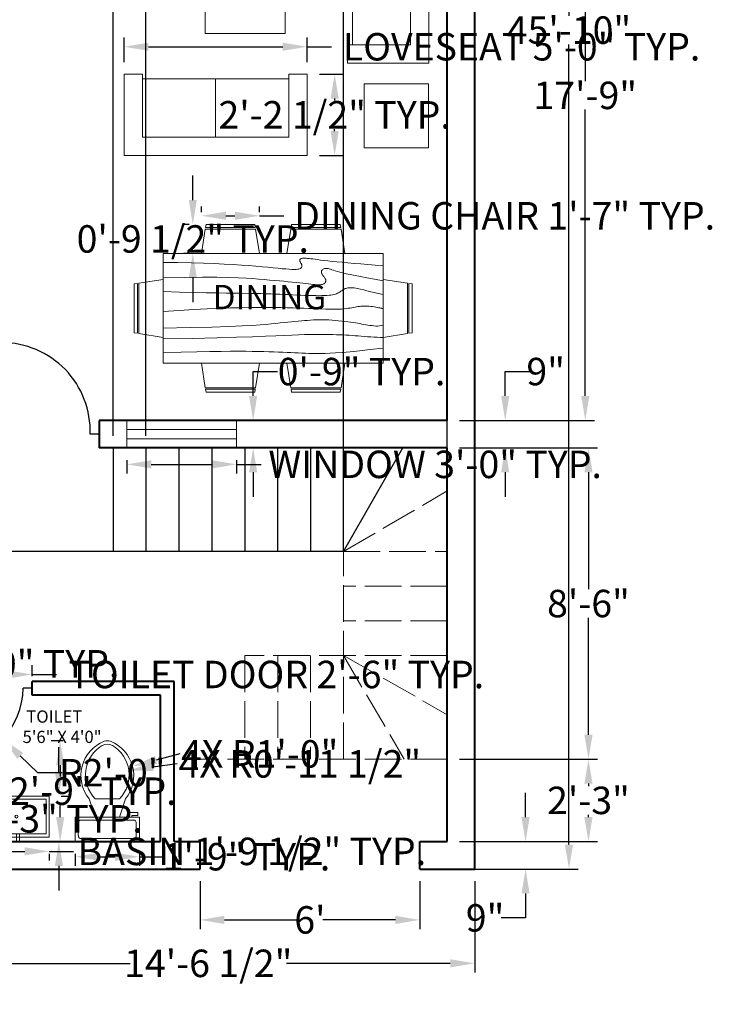
# Model space of a CAD drawing. Units: inches. Extents: x 927 to 1540, y 259 to 890.
# Tile 3 of 4: x 1265 to 1492, y 259 to 582. Entities that reach past the tile are written whole.
import ezdxf

# ---------------------------------------------------------------- set-up
doc = ezdxf.new("R2010")
doc.units = ezdxf.units.IN
doc.header["$MEASUREMENT"] = 0
doc.linetypes.add('ACAD_ISO02W100', pattern=[15, 12, -3])
for name, color, linetype, lineweight in [('A-ANNO-DIMS', 2, 'Continuous', 18), ('A-AREA-IDEN', 7, 'Continuous', 25), ('A-DOOR', 3, 'Continuous', 25), ('A-FLOR-FIXT', 9, 'Continuous', 18), ('A-FLOR-STRS', 7, 'Continuous', 25), ('A-FLOR-STRS-OVHD', 8, 'ACAD_ISO02W100', 18), ('A-FURN', 8, 'Continuous', 18), ('A-GLAZ', 4, 'Continuous', 18), ('A-WALL', 7, 'Continuous', 40)]:
    doc.layers.add(name, color=color, linetype=linetype, lineweight=lineweight)
doc.styles.get("Standard").update_dxf_attribs({"font": 'arial.ttf'})
doc.dimstyles.get("Standard").update_dxf_attribs({"dimtxt": 9, "dimasz": 8, "dimexe": 3, "dimexo": 4, "dimgap": 0.09, "dimtad": 0, "dimtih": 1, "dimtoh": 1, "dimdec": 0, "dimzin": 0, "dimdsep": 46, "dimlunit": 3, "dimtxsty": 'Standard', "dimcen": 0.09, "dimadec": 0, "dimazin": 0, "dimtfac": 1, "dimtdec": 0, "dimtofl": 0, "dimtmove": 0, "dimatfit": 3, "dimfxl": 1, "dimtolj": 1, "dimtzin": 0, "dimarcsym": 0})

# ---------------------------------------------------------------- blocks, each defined once
blk = doc.blocks.new('*D7')
at = {"layer": 'A-ANNO-DIMS', "color": 0, "lineweight": -2, "transparency": 16777216}
for p, q in [((1431.15, 320.39), (1431.15, 328.39)), ((1409.48, 312.39), (1434.15, 312.39)), ((1409.48, 303.39), (1434.15, 303.39)), ((1431.15, 295.39), (1431.15, 287.39)), ((1431.15, 287.39), (1423.15, 287.39))]:
    blk.add_line(p, q, dxfattribs=at)
at = {"layer": 'A-ANNO-DIMS', "color": 0, "lineweight": 100, "transparency": 16777216}
for points in [[(1429.81, 320.39), (1432.48, 320.39), (1431.15, 312.39)], [(1429.81, 295.39), (1432.48, 295.39), (1431.15, 303.39)]]:
    blk.add_solid(points, dxfattribs=at)
at = {"layer": 'Defpoints', "color": 0, "lineweight": 100, "transparency": 16777216}
for p in [(1405.48, 312.39), (1405.48, 303.39), (1431.15, 303.39)]:
    blk.add_point(p, dxfattribs=at)
at = {"layer": 'A-ANNO-DIMS', "color": 0, "transparency": 16777216, "insert": (1417.89, 287.39), "char_height": 9, "attachment_point": 5}
blk.add_mtext('\\A1;9"', dxfattribs=at)
blk = doc.blocks.new('*D8')
at = {"layer": 'A-ANNO-DIMS', "color": 0, "lineweight": -2, "transparency": 16777216}
for p, q in [((1418.48, 339.39), (1454.76, 339.39)), ((1451.76, 331.39), (1451.76, 330.58)), ((1451.76, 320.39), (1451.76, 321.2)), ((1418.48, 312.39), (1454.76, 312.39))]:
    blk.add_line(p, q, dxfattribs=at)
at = {"layer": 'A-ANNO-DIMS', "color": 0, "lineweight": 100, "transparency": 16777216}
for points in [[(1450.42, 331.39), (1453.09, 331.39), (1451.76, 339.39)], [(1450.42, 320.39), (1453.09, 320.39), (1451.76, 312.39)]]:
    blk.add_solid(points, dxfattribs=at)
at = {"layer": 'Defpoints', "color": 0, "lineweight": 100, "transparency": 16777216}
for p in [(1414.48, 339.39), (1451.76, 339.39), (1414.48, 312.39)]:
    blk.add_point(p, dxfattribs=at)
at = {"layer": 'A-ANNO-DIMS', "color": 0, "transparency": 16777216, "insert": (1451.76, 325.89), "char_height": 9, "attachment_point": 5}
blk.add_mtext('\\A1;2\'-3"', dxfattribs=at)
blk = doc.blocks.new('*D9')
at = {"layer": 'A-ANNO-DIMS', "color": 0, "lineweight": -2, "transparency": 16777216}
for p, q in [((1409.48, 441.39), (1454.76, 441.39)), ((1451.76, 433.39), (1451.76, 395.08)), ((1451.76, 347.39), (1451.76, 385.71)), ((1409.48, 339.39), (1454.76, 339.39))]:
    blk.add_line(p, q, dxfattribs=at)
at = {"layer": 'A-ANNO-DIMS', "color": 0, "lineweight": 100, "transparency": 16777216}
for points in [[(1450.43, 433.39), (1453.1, 433.39), (1451.76, 441.39)], [(1450.43, 347.39), (1453.1, 347.39), (1451.76, 339.39)]]:
    blk.add_solid(points, dxfattribs=at)
at = {"layer": 'Defpoints', "color": 0, "lineweight": 100, "transparency": 16777216}
for p in [(1405.48, 441.39), (1451.76, 441.39), (1405.48, 339.39)]:
    blk.add_point(p, dxfattribs=at)
at = {"layer": 'A-ANNO-DIMS', "color": 0, "transparency": 16777216, "insert": (1451.76, 390.39), "char_height": 9, "attachment_point": 5}
blk.add_mtext('\\A1;8\'-6"', dxfattribs=at)
blk = doc.blocks.new('*D10')
at = {"layer": 'A-ANNO-DIMS', "color": 0, "lineweight": -2, "transparency": 16777216}
for p, q in [((1424.47, 458.39), (1424.47, 466.39)), ((1424.47, 466.39), (1432.47, 466.39)), ((1409.48, 450.39), (1427.47, 450.39)), ((1409.48, 441.39), (1427.47, 441.39)), ((1424.47, 433.39), (1424.47, 425.39))]:
    blk.add_line(p, q, dxfattribs=at)
at = {"layer": 'A-ANNO-DIMS', "color": 0, "lineweight": 100, "transparency": 16777216}
for points in [[(1423.14, 458.39), (1425.81, 458.39), (1424.47, 450.39)], [(1423.14, 433.39), (1425.81, 433.39), (1424.47, 441.39)]]:
    blk.add_solid(points, dxfattribs=at)
at = {"layer": 'Defpoints', "color": 0, "lineweight": 100, "transparency": 16777216}
for p in [(1405.48, 450.39), (1424.47, 450.39), (1405.48, 441.39)]:
    blk.add_point(p, dxfattribs=at)
at = {"layer": 'A-ANNO-DIMS', "color": 0, "transparency": 16777216, "insert": (1437.74, 466.39), "char_height": 9, "attachment_point": 5}
blk.add_mtext('\\A1;9"', dxfattribs=at)
blk = doc.blocks.new('*D11')
at = {"layer": 'A-ANNO-DIMS', "color": 0, "lineweight": -2, "transparency": 16777216}
for p, q in [((1409.48, 663.39), (1453.72, 663.39)), ((1450.72, 655.39), (1450.72, 561.58)), ((1450.72, 458.39), (1450.72, 552.21)), ((1418.48, 450.39), (1453.72, 450.39))]:
    blk.add_line(p, q, dxfattribs=at)
at = {"layer": 'A-ANNO-DIMS', "color": 0, "lineweight": 100, "transparency": 16777216}
for points in [[(1449.39, 655.39), (1452.05, 655.39), (1450.72, 663.39)], [(1449.39, 458.39), (1452.05, 458.39), (1450.72, 450.39)]]:
    blk.add_solid(points, dxfattribs=at)
at = {"layer": 'Defpoints', "color": 0, "lineweight": 100, "transparency": 16777216}
for p in [(1405.48, 663.39), (1450.72, 663.39), (1414.48, 450.39)]:
    blk.add_point(p, dxfattribs=at)
at = {"layer": 'A-ANNO-DIMS', "color": 0, "transparency": 16777216, "insert": (1450.72, 556.89), "char_height": 9, "attachment_point": 5}
blk.add_mtext('\\A1;17\'-9"', dxfattribs=at)
blk = doc.blocks.new('*D15')
at = {"layer": 'A-ANNO-DIMS', "color": 0, "lineweight": -2, "transparency": 16777216}
for p, q in [((1324.48, 299.39), (1324.48, 283.73)), ((1396.48, 299.39), (1396.48, 283.73)), ((1332.48, 286.73), (1356.22, 286.73)), ((1388.48, 286.73), (1364.73, 286.73))]:
    blk.add_line(p, q, dxfattribs=at)
at = {"layer": 'A-ANNO-DIMS', "color": 0, "lineweight": 100, "transparency": 16777216}
for points in [[(1332.48, 288.06), (1332.48, 285.39), (1324.48, 286.73)], [(1388.48, 288.06), (1388.48, 285.39), (1396.48, 286.73)]]:
    blk.add_solid(points, dxfattribs=at)
at = {"layer": 'Defpoints', "color": 0, "lineweight": 100, "transparency": 16777216}
for p in [(1324.48, 303.39), (1396.48, 303.39), (1396.48, 286.73)]:
    blk.add_point(p, dxfattribs=at)
at = {"layer": 'A-ANNO-DIMS', "color": 0, "transparency": 16777216, "insert": (1360.48, 286.73), "char_height": 9, "attachment_point": 5}
blk.add_mtext("\\A1;6'", dxfattribs=at)
blk = doc.blocks.new('DOOR-SINGLE-36-OPENING')
for p, q in [((3, 0), (3, 30)), ((3, 30), (4, 30)), ((4, 30), (4, 0)), ((0, 0), (3, 0)), ((4, 0), (3, 0)), ((36, 0), (33, 0))]:
    blk.add_line(p, q)
blk.add_arc((4, 0.98), 29.02, 358.058, 90)
blk = doc.blocks.new('DOOR-SINGLE-30-OPENING')
for p, q in [((0, 24), (3, 24)), ((3, 24), (3, 0)), ((4, 24), (3, 24)), ((4, 0), (4, 24)), ((30, 24), (27, 24)), ((3, 0), (4, 0))]:
    blk.add_line(p, q)
blk.add_arc((2.98, 24), 24.02, 272.4378, 0)
blk = doc.blocks.new('SOFA-LOVESEAT-60')
for p, q in [((26.6182, 60.00004), (26.6182, 0)), ((0, 54.00004), (1.558, 54.00004)), ((1.558, 54.00004), (1.558, 6)), ((1.558, 54.00004), (20.6182, 53.99984)), ((20.6182, 53.99984), (20.6182, 6.00018)), ((1.558, 30.00004), (20.6182, 30.00004)), ((0, 6), (1.558, 6)), ((20.6182, 6.00018), (1.558, 6))]:
    blk.add_line(p, q)
for points in [[(0, 54.00004), (0, 60.00004), (26.6182, 60.00004)], [(26.6182, 0), (0, 0), (0, 6)]]:
    blk.add_lwpolyline(points)
blk = doc.blocks.new('CHAIR-DINING')
for p, q in [((1.2504, 8.00297), (0, 0)), ((1.2543, 8.00238), (17.7239, 8.00238)), ((1.4847, 9.50238), (1.3285, 8.5028)), ((17.6431, 8.50238), (1.3313, 8.50238)), ((1.4847, 9.50238), (17.4847, 9.50238)), ((17.641, 8.50204), (17.4847, 9.50238)), ((18.9695, 0), (17.7192, 8.00164))]:
    blk.add_line(p, q)
blk = doc.blocks.new('WC-TANK-TYPE')
for p, q in [((23.5, 17.5), (23.5, 20.5)), ((23.5, 20.5), (24.5, 20.5)), ((24.5, 20.5), (24.5, 18.5)), ((25, 14.5), (19, 16.5)), ((25, 17.5), (23.5, 17.5)), ((24.5, 18.5), (25, 18.5)), ((19, 6.5), (19, 14.5)), ((25, 6.5), (19, 4.5)), ((27, 1), (31, 1))]:
    blk.add_line(p, q)
blk.add_lwpolyline([(25, 0), (33, 0), (33, 21), (25, 21)], close=True)
for points in [[(31, 20), (27, 20)], [(26, 19), (26, 2)], [(32, 2), (32, 19)]]:
    blk.add_lwpolyline(points)
for centre, radius, start, end in [((26.87, 19.12), 0.884, 81.8699, 188.1301), ((31.12, 19.12), 0.884, 351.8699, 98.1301), ((11.42, 6.98), 12.17, 51.4691, 157.9714), ((11.18, 6.3), 11.33, 46.3677, 148.9468), ((4, 10.5), 4, 164.8605, 195.1395), ((5.12, 10.5), 4, 155.7318, 204.2682), ((11.42, 14.02), 12.17, 202.0284, 308.5307), ((11.18, 14.7), 11.33, 211.053, 313.6321), ((26.87, 1.88), 0.884, 171.8699, 278.1301), ((31.12, 1.88), 0.884, 261.8699, 8.1301)]:
    blk.add_arc(centre, radius, start, end)
blk = doc.blocks.new('LAVATORY-RECTANGULAR')
for p, q in [((10.69, 2.5), (10.69, 0)), ((11.69, 2.5), (11.69, 0))]:
    blk.add_line(p, q)
for points in [[(0, 1.5), (21.39, 1.5), (21.39, 14.9), (0, 14.9)], [(1, 2.5), (20.39, 2.5), (20.39, 13.9), (1, 13.9)]]:
    blk.add_lwpolyline(points, close=True)
blk.add_circle((10.69, 8.2), 0.491)
blk = doc.blocks.new('WINDOW-36')
for p, q in [((0, 9), (0, 0)), ((36, 9), (36, 0)), ((0, 6), (36, 6)), ((0, 3), (36, 3))]:
    blk.add_line(p, q)
blk = doc.blocks.new('*D30')
at = {"layer": 'A-ANNO-DIMS', "color": 0, "lineweight": -2, "transparency": 16777216}
for p, q in [((1324.96, 518.6), (1324.96, 520.44)), ((1343.93, 518.6), (1343.93, 520.44)), ((1332.96, 517.44), (1335.93, 517.44)), ((1343.93, 517.44), (1351.93, 517.44))]:
    blk.add_line(p, q, dxfattribs=at)
at = {"layer": 'A-ANNO-DIMS', "color": 0, "lineweight": 100, "transparency": 16777216}
for points in [[(1332.96, 518.78), (1332.96, 516.11), (1324.96, 517.44)], [(1335.93, 518.78), (1335.93, 516.11), (1343.93, 517.44)]]:
    blk.add_solid(points, dxfattribs=at)
at = {"layer": 'Defpoints', "color": 0, "lineweight": 100, "transparency": 16777216}
for p in [(1343.93, 517.44), (1324.96, 514.6), (1343.93, 514.6)]:
    blk.add_point(p, dxfattribs=at)
at = {"layer": 'A-ANNO-DIMS', "color": 0, "transparency": 16777216, "insert": (1424.28, 517.44), "char_height": 9, "attachment_point": 5}
blk.add_mtext('\\A1;DINING CHAIR 1\'-7" TYP.', dxfattribs=at)
blk = doc.blocks.new('*D31')
at = {"layer": 'A-ANNO-DIMS', "color": 0, "lineweight": -2, "transparency": 16777216}
for p, q in [((1322.11, 522.6), (1322.11, 530.6)), ((1320.96, 514.6), (1319.11, 514.6)), ((1320.96, 505.1), (1319.11, 505.1)), ((1322.11, 497.1), (1322.11, 489.1))]:
    blk.add_line(p, q, dxfattribs=at)
at = {"layer": 'A-ANNO-DIMS', "color": 0, "lineweight": 100, "transparency": 16777216}
for points in [[(1320.78, 522.6), (1323.44, 522.6), (1322.11, 514.6)], [(1320.78, 497.1), (1323.44, 497.1), (1322.11, 505.1)]]:
    blk.add_solid(points, dxfattribs=at)
at = {"layer": 'Defpoints', "color": 0, "lineweight": 100, "transparency": 16777216}
for p in [(1322.11, 514.6), (1324.96, 514.6), (1324.96, 505.1)]:
    blk.add_point(p, dxfattribs=at)
at = {"layer": 'A-ANNO-DIMS', "color": 0, "transparency": 16777216, "insert": (1322.11, 509.85), "char_height": 9, "attachment_point": 5}
blk.add_mtext('\\A1;0\'-9 1/2" TYP.', dxfattribs=at)
blk = doc.blocks.new('*D34')
at = {"layer": 'A-ANNO-DIMS', "color": 0, "lineweight": -2, "transparency": 16777216}
for p, q in [((1239.48, 366.64), (1239.48, 370.14)), ((1269.48, 366.64), (1269.48, 370.14)), ((1247.48, 367.14), (1261.48, 367.14)), ((1269.48, 367.14), (1277.48, 367.14))]:
    blk.add_line(p, q, dxfattribs=at)
at = {"layer": 'A-ANNO-DIMS', "color": 0, "lineweight": 100, "transparency": 16777216}
for points in [[(1247.48, 368.47), (1247.48, 365.81), (1239.48, 367.14)], [(1261.48, 368.47), (1261.48, 365.81), (1269.48, 367.14)]]:
    blk.add_solid(points, dxfattribs=at)
at = {"layer": 'Defpoints', "color": 0, "lineweight": 100, "transparency": 16777216}
for p in [(1269.48, 367.14), (1239.48, 362.64), (1269.48, 362.64)]:
    blk.add_point(p, dxfattribs=at)
at = {"layer": 'A-ANNO-DIMS', "color": 0, "transparency": 16777216, "insert": (1349.47, 367.14), "char_height": 9, "attachment_point": 5}
blk.add_mtext('\\A1;TOILET DOOR 2\'-6" TYP.', dxfattribs=at)
blk = doc.blocks.new('*D35')
at = {"layer": 'A-ANNO-DIMS', "color": 0, "lineweight": -2, "transparency": 16777216}
for p, q in [((1234.98, 362.64), (1234.98, 370.64)), ((1234.98, 370.64), (1242.98, 370.64)), ((1235.48, 362.64), (1231.98, 362.64)), ((1234.98, 346.64), (1234.98, 354.64)), ((1235.48, 338.64), (1231.98, 338.64))]:
    blk.add_line(p, q, dxfattribs=at)
at = {"layer": 'A-ANNO-DIMS', "color": 0, "lineweight": 100, "transparency": 16777216}
for points in [[(1233.64, 354.64), (1236.31, 354.64), (1234.98, 362.64)], [(1233.64, 346.64), (1236.31, 346.64), (1234.98, 338.64)]]:
    blk.add_solid(points, dxfattribs=at)
at = {"layer": 'Defpoints', "color": 0, "lineweight": 100, "transparency": 16777216}
for p in [(1234.98, 362.64), (1239.48, 362.64), (1239.48, 338.64)]:
    blk.add_point(p, dxfattribs=at)
at = {"layer": 'A-ANNO-DIMS', "color": 0, "transparency": 16777216, "insert": (1270.57, 370.64), "char_height": 9, "attachment_point": 5}
blk.add_mtext('\\A1;2\'-0" TYP.', dxfattribs=at)
blk = doc.blocks.new('*D36')
at = {"layer": 'A-ANNO-DIMS', "color": 0, "lineweight": -2, "transparency": 16777216}
for p, q in [((1299.59, 567.82), (1299.59, 575.82)), ((1359.59, 567.82), (1359.59, 575.82)), ((1307.59, 572.82), (1351.59, 572.82)), ((1359.59, 572.82), (1367.59, 572.82))]:
    blk.add_line(p, q, dxfattribs=at)
at = {"layer": 'A-ANNO-DIMS', "color": 0, "lineweight": 100, "transparency": 16777216}
for points in [[(1307.59, 574.16), (1307.59, 571.49), (1299.59, 572.82)], [(1351.59, 574.16), (1351.59, 571.49), (1359.59, 572.82)]]:
    blk.add_solid(points, dxfattribs=at)
at = {"layer": 'Defpoints', "color": 0, "lineweight": 100, "transparency": 16777216}
for p in [(1359.59, 572.82), (1299.59, 563.82), (1359.59, 563.82)]:
    blk.add_point(p, dxfattribs=at)
at = {"layer": 'A-ANNO-DIMS', "color": 0, "transparency": 16777216, "insert": (1429.85, 572.82), "char_height": 9, "attachment_point": 5}
blk.add_mtext('\\A1;LOVESEAT 5\'-0" TYP.', dxfattribs=at)
blk = doc.blocks.new('*D37')
at = {"layer": 'A-ANNO-DIMS', "color": 0, "lineweight": -2, "transparency": 16777216}
for p, q in [((1363.59, 563.82), (1371.59, 563.82)), ((1368.59, 555.82), (1368.59, 555.26)), ((1368.59, 545.21), (1368.59, 545.77)), ((1363.59, 537.21), (1371.59, 537.21))]:
    blk.add_line(p, q, dxfattribs=at)
at = {"layer": 'A-ANNO-DIMS', "color": 0, "lineweight": 100, "transparency": 16777216}
for points in [[(1367.26, 555.82), (1369.93, 555.82), (1368.59, 563.82)], [(1367.26, 545.21), (1369.93, 545.21), (1368.59, 537.21)]]:
    blk.add_solid(points, dxfattribs=at)
at = {"layer": 'Defpoints', "color": 0, "lineweight": 100, "transparency": 16777216}
for p in [(1359.59, 563.82), (1359.59, 537.21), (1368.59, 537.21)]:
    blk.add_point(p, dxfattribs=at)
at = {"layer": 'A-ANNO-DIMS', "color": 0, "transparency": 16777216, "insert": (1368.59, 550.52), "char_height": 9, "attachment_point": 5}
blk.add_mtext('\\A1;2\'-2 1/2" TYP.', dxfattribs=at)
blk = doc.blocks.new('*D44')
at = {"layer": 'A-ANNO-DIMS', "color": 0, "lineweight": -2, "transparency": 16777216}
for p, q in [((1279.6, 345.44), (1275.65, 345.44)), ((1278.65, 337.44), (1278.65, 333.66)), ((1278.65, 320.39), (1278.65, 324.17)), ((1279.6, 312.39), (1275.65, 312.39))]:
    blk.add_line(p, q, dxfattribs=at)
at = {"layer": 'A-ANNO-DIMS', "color": 0, "lineweight": 100, "transparency": 16777216}
for points in [[(1277.31, 337.44), (1279.98, 337.44), (1278.65, 345.44)], [(1277.31, 320.39), (1279.98, 320.39), (1278.65, 312.39)]]:
    blk.add_solid(points, dxfattribs=at)
at = {"layer": 'Defpoints', "color": 0, "lineweight": 100, "transparency": 16777216}
for p in [(1283.6, 345.44), (1278.65, 312.39), (1283.6, 312.39)]:
    blk.add_point(p, dxfattribs=at)
at = {"layer": 'A-ANNO-DIMS', "color": 0, "transparency": 16777216, "insert": (1278.65, 328.91), "char_height": 9, "attachment_point": 5}
blk.add_mtext('\\A1;WC 2\'-9" TYP.', dxfattribs=at)
blk = doc.blocks.new('*D45')
at = {"layer": 'A-ANNO-DIMS', "color": 0, "lineweight": -2, "transparency": 16777216}
for p, q in [((1283.6, 308.39), (1283.6, 304.43)), ((1291.6, 307.43), (1296.6, 307.43)), ((1304.6, 308.39), (1304.6, 304.43)), ((1304.6, 307.43), (1312.6, 307.43))]:
    blk.add_line(p, q, dxfattribs=at)
at = {"layer": 'A-ANNO-DIMS', "color": 0, "lineweight": 100, "transparency": 16777216}
for points in [[(1291.6, 308.77), (1291.6, 306.1), (1283.6, 307.43)], [(1296.6, 308.77), (1296.6, 306.1), (1304.6, 307.43)]]:
    blk.add_solid(points, dxfattribs=at)
at = {"layer": 'Defpoints', "color": 0, "lineweight": 100, "transparency": 16777216}
for p in [(1283.6, 312.39), (1304.6, 312.39), (1304.6, 307.43)]:
    blk.add_point(p, dxfattribs=at)
at = {"layer": 'A-ANNO-DIMS', "color": 0, "transparency": 16777216, "insert": (1339.7, 307.43), "char_height": 9, "attachment_point": 5}
blk.add_mtext('\\A1;1\'-9" TYP.', dxfattribs=at)
blk = doc.blocks.new('*D46')
at = {"layer": 'A-ANNO-DIMS', "color": 0, "lineweight": -2, "transparency": 16777216}
for p, q in [((1253.64, 308.39), (1253.64, 306.18)), ((1261.64, 309.18), (1267.03, 309.18)), ((1275.03, 309.18), (1283.03, 309.18)), ((1275.03, 308.39), (1275.03, 306.18))]:
    blk.add_line(p, q, dxfattribs=at)
at = {"layer": 'A-ANNO-DIMS', "color": 0, "lineweight": 100, "transparency": 16777216}
for points in [[(1261.64, 310.52), (1261.64, 307.85), (1253.64, 309.18)], [(1267.03, 310.52), (1267.03, 307.85), (1275.03, 309.18)]]:
    blk.add_solid(points, dxfattribs=at)
at = {"layer": 'Defpoints', "color": 0, "lineweight": 100, "transparency": 16777216}
for p in [(1253.64, 312.39), (1275.03, 312.39), (1275.03, 309.18)]:
    blk.add_point(p, dxfattribs=at)
at = {"layer": 'A-ANNO-DIMS', "color": 0, "transparency": 16777216, "insert": (1341.45, 309.18), "char_height": 9, "attachment_point": 5}
blk.add_mtext('\\A1;BASIN 1\'-9 1/2" TYP.', dxfattribs=at)
blk = doc.blocks.new('*D47')
at = {"layer": 'A-ANNO-DIMS', "color": 0, "lineweight": -2, "transparency": 16777216}
for p, q in [((1278.23, 335.29), (1278.23, 343.29)), ((1279.03, 327.29), (1281.23, 327.29)), ((1279.03, 312.39), (1281.23, 312.39)), ((1278.23, 304.39), (1278.23, 296.39))]:
    blk.add_line(p, q, dxfattribs=at)
at = {"layer": 'A-ANNO-DIMS', "color": 0, "lineweight": 100, "transparency": 16777216}
for points in [[(1276.9, 335.29), (1279.57, 335.29), (1278.23, 327.29)], [(1276.9, 304.39), (1279.57, 304.39), (1278.23, 312.39)]]:
    blk.add_solid(points, dxfattribs=at)
at = {"layer": 'Defpoints', "color": 0, "lineweight": 100, "transparency": 16777216}
for p in [(1275.03, 327.29), (1278.23, 327.29), (1275.03, 312.39)]:
    blk.add_point(p, dxfattribs=at)
at = {"layer": 'A-ANNO-DIMS', "color": 0, "transparency": 16777216, "insert": (1278.23, 319.84), "char_height": 9, "attachment_point": 5}
blk.add_mtext('\\A1;1\'-3" TYP.', dxfattribs=at)
blk = doc.blocks.new('*D48')
at = {"layer": 'A-ANNO-DIMS', "color": 0, "lineweight": -2, "transparency": 16777216}
for p, q in [((1300.48, 437.39), (1300.48, 432.99)), ((1308.48, 435.99), (1328.48, 435.99)), ((1336.48, 437.39), (1336.48, 432.99)), ((1336.48, 435.99), (1344.48, 435.99))]:
    blk.add_line(p, q, dxfattribs=at)
at = {"layer": 'A-ANNO-DIMS', "color": 0, "lineweight": 100, "transparency": 16777216}
for points in [[(1308.48, 437.32), (1308.48, 434.66), (1300.48, 435.99)], [(1328.48, 437.32), (1328.48, 434.66), (1336.48, 435.99)]]:
    blk.add_solid(points, dxfattribs=at)
at = {"layer": 'Defpoints', "color": 0, "lineweight": 100, "transparency": 16777216}
for p in [(1300.48, 441.39), (1336.48, 441.39), (1336.48, 435.99)]:
    blk.add_point(p, dxfattribs=at)
at = {"layer": 'A-ANNO-DIMS', "color": 0, "transparency": 16777216, "insert": (1401.51, 435.99), "char_height": 9, "attachment_point": 5}
blk.add_mtext('\\A1;WINDOW 3\'-0" TYP.', dxfattribs=at)
blk = doc.blocks.new('*D49')
at = {"layer": 'A-ANNO-DIMS', "color": 0, "lineweight": -2, "transparency": 16777216}
for p, q in [((1341.88, 458.39), (1341.88, 466.39)), ((1341.88, 466.39), (1349.88, 466.39)), ((1340.48, 450.39), (1344.88, 450.39)), ((1340.48, 441.39), (1344.88, 441.39)), ((1341.88, 433.39), (1341.88, 425.39))]:
    blk.add_line(p, q, dxfattribs=at)
at = {"layer": 'A-ANNO-DIMS', "color": 0, "lineweight": 100, "transparency": 16777216}
for points in [[(1340.54, 458.39), (1343.21, 458.39), (1341.88, 450.39)], [(1340.54, 433.39), (1343.21, 433.39), (1341.88, 441.39)]]:
    blk.add_solid(points, dxfattribs=at)
at = {"layer": 'Defpoints', "color": 0, "lineweight": 100, "transparency": 16777216}
for p in [(1336.48, 450.39), (1341.88, 450.39), (1336.48, 441.39)]:
    blk.add_point(p, dxfattribs=at)
at = {"layer": 'A-ANNO-DIMS', "color": 0, "transparency": 16777216, "insert": (1377.4, 466.39), "char_height": 9, "attachment_point": 5}
blk.add_mtext('\\A1;0\'-9" TYP.', dxfattribs=at)
blk = doc.blocks.new('*D51')
at = {"layer": 'A-ANNO-DIMS', "color": 0, "lineweight": -2, "transparency": 16777216}
for p, q in [((1418.48, 853.14), (1448.38, 853.14)), ((1445.38, 845.14), (1445.38, 582.95)), ((1445.38, 311.39), (1445.38, 573.58)), ((1418.48, 303.39), (1448.38, 303.39))]:
    blk.add_line(p, q, dxfattribs=at)
at = {"layer": 'A-ANNO-DIMS', "color": 0, "lineweight": 100, "transparency": 16777216}
for points in [[(1444.04, 845.14), (1446.71, 845.14), (1445.38, 853.14)], [(1444.04, 311.39), (1446.71, 311.39), (1445.38, 303.39)]]:
    blk.add_solid(points, dxfattribs=at)
at = {"layer": 'Defpoints', "color": 0, "lineweight": 100, "transparency": 16777216}
for p in [(1414.48, 853.14), (1445.38, 853.14), (1414.48, 303.39)]:
    blk.add_point(p, dxfattribs=at)
at = {"layer": 'A-ANNO-DIMS', "color": 0, "transparency": 16777216, "insert": (1445.38, 578.27), "char_height": 9, "attachment_point": 5}
blk.add_mtext('\\A1;45\'-10"', dxfattribs=at)
blk = doc.blocks.new('*D52')
at = {"layer": 'A-ANNO-DIMS', "color": 0, "lineweight": -2, "transparency": 16777216}
for p, q in [((1239.89, 299.39), (1239.89, 269.49)), ((1414.48, 299.39), (1414.48, 269.49)), ((1247.89, 272.49), (1301.57, 272.49)), ((1406.48, 272.49), (1352.79, 272.49))]:
    blk.add_line(p, q, dxfattribs=at)
at = {"layer": 'A-ANNO-DIMS', "color": 0, "lineweight": 100, "transparency": 16777216}
for points in [[(1247.89, 273.82), (1247.89, 271.16), (1239.89, 272.49)], [(1406.48, 273.82), (1406.48, 271.16), (1414.48, 272.49)]]:
    blk.add_solid(points, dxfattribs=at)
at = {"layer": 'Defpoints', "color": 0, "lineweight": 100, "transparency": 16777216}
for p in [(1239.89, 303.39), (1414.48, 303.39), (1414.48, 272.49)]:
    blk.add_point(p, dxfattribs=at)
at = {"layer": 'A-ANNO-DIMS', "color": 0, "transparency": 16777216, "insert": (1327.18, 272.49), "char_height": 9, "attachment_point": 5}
blk.add_mtext('\\A1;14\'-6 1/2"', dxfattribs=at)
blk = doc.blocks.new('*D54')
at = {"layer": 'A-ANNO-DIMS', "color": 0, "lineweight": -2, "transparency": 16777216}
for p, q in [((1363.48, 884.04), (1355.48, 884.04)), ((1371.48, 411.39), (1371.48, 887.04)), ((1405.48, 411.39), (1405.48, 887.04)), ((1413.48, 884.04), (1421.48, 884.04))]:
    blk.add_line(p, q, dxfattribs=at)
at = {"layer": 'A-ANNO-DIMS', "color": 0, "lineweight": 100, "transparency": 16777216}
for points in [[(1363.48, 885.38), (1363.48, 882.71), (1371.48, 884.04)], [(1413.48, 885.38), (1413.48, 882.71), (1405.48, 884.04)]]:
    blk.add_solid(points, dxfattribs=at)
at = {"layer": 'Defpoints', "color": 0, "lineweight": 100, "transparency": 16777216}
for p in [(1405.48, 884.04), (1371.48, 407.39), (1405.48, 407.39)]:
    blk.add_point(p, dxfattribs=at)
at = {"layer": 'A-ANNO-DIMS', "color": 0, "transparency": 16777216, "insert": (1388.48, 884.04), "char_height": 9, "attachment_point": 5}
blk.add_mtext('\\A1;2\'-10"', dxfattribs=at)
blk = doc.blocks.new('*D55')
at = {"layer": 'A-ANNO-DIMS', "color": 0, "lineweight": -2, "transparency": 16777216}
for p, q in [((1287.98, 884.04), (1279.98, 884.04)), ((1295.98, 445.39), (1295.98, 887.04)), ((1306.76, 445.39), (1306.76, 887.04)), ((1314.76, 884.04), (1322.76, 884.04))]:
    blk.add_line(p, q, dxfattribs=at)
at = {"layer": 'A-ANNO-DIMS', "color": 0, "lineweight": 100, "transparency": 16777216}
for points in [[(1287.98, 885.38), (1287.98, 882.71), (1295.98, 884.04)], [(1314.76, 885.38), (1314.76, 882.71), (1306.76, 884.04)]]:
    blk.add_solid(points, dxfattribs=at)
at = {"layer": 'Defpoints', "color": 0, "lineweight": 100, "transparency": 16777216}
for p in [(1306.76, 884.04), (1295.98, 441.39), (1306.76, 441.39)]:
    blk.add_point(p, dxfattribs=at)
at = {"layer": 'A-ANNO-DIMS', "color": 0, "transparency": 16777216, "insert": (1338.31, 884.04), "char_height": 9, "attachment_point": 5}
blk.add_mtext('\\A1;0\'-11"', dxfattribs=at)
blk = doc.blocks.new('*D60')
at = {"layer": 'A-ANNO-DIMS', "color": 0, "lineweight": -2, "transparency": 16777216}
for p, q in [((1242.37, 362.64), (1242.55, 362.64)), ((1242.46, 362.55), (1242.46, 362.73)), ((1271.35, 334.95), (1265.58, 340.49)), ((1279.35, 334.95), (1271.35, 334.95))]:
    blk.add_line(p, q, dxfattribs=at)
at = {"layer": 'A-ANNO-DIMS', "color": 0, "lineweight": 100, "transparency": 16777216}
blk.add_solid([(1266.5, 341.45), (1264.65, 339.52), (1259.8, 346.02)], dxfattribs=at)
at = {"layer": 'Defpoints', "color": 0, "lineweight": 100, "transparency": 16777216}
for p in [(1242.46, 362.64), (1259.8, 346.02)]:
    blk.add_point(p, dxfattribs=at)
at = {"layer": 'A-ANNO-DIMS', "color": 0, "transparency": 16777216, "insert": (1295.71, 334.95), "char_height": 9, "attachment_point": 5}
blk.add_mtext('\\A1;R2\'-0"', dxfattribs=at)
blk = doc.blocks.new('*D61')
at = {"layer": 'A-ANNO-DIMS', "color": 0, "lineweight": -2, "transparency": 16777216}
for p, q in [((1317.83, 341.13), (1310.09, 339.1)), ((1290.49, 333.97), (1290.67, 333.97)), ((1290.58, 333.88), (1290.58, 334.06))]:
    blk.add_line(p, q, dxfattribs=at)
at = {"layer": 'A-ANNO-DIMS', "color": 0, "lineweight": 100, "transparency": 16777216}
blk.add_solid([(1309.75, 340.39), (1310.43, 337.81), (1302.35, 337.06)], dxfattribs=at)
at = {"layer": 'Defpoints', "color": 0, "lineweight": 100, "transparency": 16777216}
for p in [(1302.35, 337.06), (1290.58, 333.97)]:
    blk.add_point(p, dxfattribs=at)
at = {"layer": 'A-ANNO-DIMS', "color": 0, "transparency": 16777216, "insert": (1344.04, 341.13), "char_height": 9, "attachment_point": 5}
blk.add_mtext('\\A1;4X R1\'-0"', dxfattribs=at)
blk = doc.blocks.new('*D62')
at = {"layer": 'A-ANNO-DIMS', "color": 0, "lineweight": -2, "transparency": 16777216}
for p, q in [((1316.99, 337.85), (1309.06, 336.78)), ((1289.81, 334.21), (1289.99, 334.21)), ((1289.9, 334.12), (1289.9, 334.3))]:
    blk.add_line(p, q, dxfattribs=at)
at = {"layer": 'A-ANNO-DIMS', "color": 0, "lineweight": 100, "transparency": 16777216}
blk.add_solid([(1308.88, 338.11), (1309.24, 335.46), (1301.13, 335.72)], dxfattribs=at)
at = {"layer": 'Defpoints', "color": 0, "lineweight": 100, "transparency": 16777216}
for p in [(1301.13, 335.72), (1289.9, 334.21)]:
    blk.add_point(p, dxfattribs=at)
at = {"layer": 'A-ANNO-DIMS', "color": 0, "transparency": 16777216, "insert": (1357.18, 337.85), "char_height": 9, "attachment_point": 5}
blk.add_mtext('\\A1;4X R0\'-11 1/2"', dxfattribs=at)

msp = doc.modelspace()

# ---------------------------------------------------------------- linework, layer by layer
at = {"layer": 'A-FLOR-STRS'}
for p, q in [((1291.48, 441.39), (1295.98, 441.39)), ((1295.98, 441.39), (1295.98, 407.39)), ((1306.76, 441.39), (1306.76, 407.39)), ((1317.55, 441.39), (1317.55, 407.39)), ((1328.33, 441.39), (1328.33, 407.39)), ((1339.12, 441.39), (1339.12, 407.39)), ((1349.91, 441.39), (1349.91, 407.39)), ((1360.69, 441.39), (1360.69, 407.39)), ((1371.48, 407.39), (1390.9, 441.39)), ((1371.48, 407.39), (1371.48, 441.39)), ((1371.48, 407.39), (1198.54, 407.39))]:
    msp.add_line(p, q, dxfattribs=at)
at = {"layer": 'A-FLOR-STRS-OVHD'}
for p, q in [((1371.48, 407.39), (1405.48, 427.28)), ((1371.48, 339.39), (1371.48, 407.39)), ((1371.48, 407.39), (1405.48, 407.39)), ((1405.48, 396.05), (1371.48, 396.05)), ((1405.48, 384.72), (1371.48, 384.72)), ((1405.48, 373.39), (1339.16, 373.39)), ((1339.16, 373.39), (1339.16, 339.39)), ((1349.94, 373.39), (1349.94, 339.39)), ((1360.73, 373.39), (1360.73, 339.39)), ((1371.48, 373.39), (1391.36, 339.39)), ((1371.48, 373.39), (1405.48, 353.97)), ((1405.48, 339.39), (1315.98, 339.39))]:
    msp.add_line(p, q, dxfattribs=at)
at = {"layer": 'A-FURN'}
for p, q in [((1384.44, 505.1), (1312.44, 505.1)), ((1312.44, 505.1), (1312.44, 469.1)), ((1384.44, 469.1), (1384.44, 505.1)), ((1312.44, 469.1), (1384.44, 469.1))]:
    msp.add_line(p, q, dxfattribs=at)
for points in [[(1352.35, 577.18), (1326.12, 577.18), (1326.12, 622.34), (1352.35, 622.34)], [(1399.3, 560.68), (1378.3, 560.68), (1378.3, 539.68), (1399.3, 539.68)]]:
    msp.add_lwpolyline(points, close=True, dxfattribs=at)
for points in [[(1312.44, 502.1), (1317.26, 502.08), (1321.63, 502.01), (1325.59, 501.91), (1329.16, 501.79), (1332.4, 501.63), (1335.34, 501.46), (1338.02, 501.28), (1340.48, 501.1), (1342.75, 500.91), (1344.84, 500.73), (1346.75, 500.55), (1348.48, 500.39), (1350.04, 500.24), (1351.42, 500.11), (1352.64, 500.01), (1353.69, 499.93), (1354.58, 499.88), (1355.32, 499.87), (1355.93, 499.88), (1356.42, 499.91), (1356.81, 499.97), (1357.11, 500.05), (1357.35, 500.15), (1357.52, 500.26), (1357.66, 500.4), (1357.76, 500.54), (1357.83, 500.7), (1357.87, 500.86), (1357.88, 501.02), (1357.86, 501.19), (1357.83, 501.35), (1357.77, 501.51), (1357.7, 501.67), (1357.62, 501.81), (1357.54, 501.95), (1357.45, 502.09), (1357.37, 502.22), (1357.29, 502.35), (1357.23, 502.47), (1357.19, 502.6), (1357.17, 502.72), (1357.18, 502.84), (1357.2, 502.96), (1357.25, 503.08), (1357.33, 503.18), (1357.43, 503.28), (1357.55, 503.36), (1357.69, 503.43), (1357.86, 503.49), (1358.06, 503.52), (1358.29, 503.55), (1358.57, 503.56), (1358.89, 503.55), (1359.26, 503.52), (1359.69, 503.49), (1360.19, 503.43), (1360.76, 503.36), (1361.41, 503.28), (1362.16, 503.18), (1363.01, 503.07), (1363.98, 502.94), (1365.08, 502.81), (1366.33, 502.67), (1367.73, 502.51), (1369.3, 502.35), (1371.03, 502.19), (1372.91, 502.01), (1374.95, 501.84), (1377.12, 501.66), (1379.43, 501.47), (1381.88, 501.28), (1384.44, 501.1)], [(1312.44, 497.1), (1319.46, 497.24), (1325.27, 497.3), (1330.02, 497.3), (1333.87, 497.23), (1337, 497.13), (1339.56, 496.99), (1341.73, 496.84), (1343.65, 496.68), (1345.47, 496.53), (1347.22, 496.38), (1348.88, 496.24), (1350.47, 496.11), (1351.97, 495.98), (1353.38, 495.85), (1354.71, 495.72), (1355.94, 495.6), (1357.08, 495.47), (1358.13, 495.35), (1359.09, 495.24), (1359.97, 495.13), (1360.77, 495.03), (1361.48, 494.95), (1362.12, 494.89), (1362.69, 494.85), (1363.19, 494.83), (1363.62, 494.83), (1363.99, 494.85), (1364.32, 494.9), (1364.59, 494.96), (1364.82, 495.05), (1365.02, 495.15), (1365.19, 495.26), (1365.34, 495.4), (1365.45, 495.54), (1365.55, 495.7), (1365.62, 495.87), (1365.66, 496.04), (1365.67, 496.23), (1365.65, 496.41), (1365.61, 496.6), (1365.53, 496.79), (1365.43, 496.97), (1365.31, 497.16), (1365.17, 497.35), (1365.03, 497.54), (1364.88, 497.72), (1364.74, 497.91), (1364.61, 498.1), (1364.49, 498.28), (1364.39, 498.47), (1364.32, 498.66), (1364.26, 498.84), (1364.24, 499.01), (1364.24, 499.19), (1364.28, 499.35), (1364.36, 499.51), (1364.47, 499.67), (1364.62, 499.81), (1364.8, 499.93), (1365.01, 500.04), (1365.25, 500.12), (1365.52, 500.17), (1365.8, 500.19), (1366.11, 500.18), (1366.43, 500.13), (1366.78, 500.04), (1367.18, 499.93), (1367.63, 499.78), (1368.16, 499.61), (1368.77, 499.41), (1369.49, 499.2), (1370.32, 498.97), (1371.28, 498.73), (1372.4, 498.47), (1373.72, 498.18), (1375.27, 497.86), (1377.08, 497.5), (1379.19, 497.09), (1381.63, 496.63), (1384.44, 496.1)], [(1312.44, 492.6), (1317.72, 492.43), (1322.37, 492.31), (1326.45, 492.22), (1330.01, 492.15), (1333.14, 492.1), (1335.89, 492.07), (1338.33, 492.04), (1340.52, 492.01), (1342.53, 491.98), (1344.38, 491.94), (1346.1, 491.89), (1347.7, 491.84), (1349.21, 491.78), (1350.66, 491.72), (1352.06, 491.66), (1353.44, 491.6), (1354.81, 491.54), (1356.18, 491.48), (1357.51, 491.42), (1358.82, 491.37), (1360.07, 491.33), (1361.27, 491.29), (1362.4, 491.27), (1363.44, 491.26), (1364.39, 491.27), (1365.26, 491.3), (1366.04, 491.33), (1366.74, 491.39), (1367.37, 491.46), (1367.93, 491.55), (1368.42, 491.65), (1368.86, 491.76), (1369.24, 491.9), (1369.57, 492.04), (1369.87, 492.2), (1370.13, 492.36), (1370.37, 492.52), (1370.59, 492.69), (1370.81, 492.85), (1371.02, 493.01), (1371.25, 493.17), (1371.48, 493.31), (1371.73, 493.44), (1371.99, 493.56), (1372.28, 493.66), (1372.58, 493.74), (1372.91, 493.8), (1373.27, 493.85), (1373.66, 493.87), (1374.08, 493.86), (1374.53, 493.84), (1374.99, 493.8), (1375.48, 493.73), (1375.98, 493.65), (1376.5, 493.55), (1377.02, 493.43), (1377.56, 493.3), (1378.15, 493.14), (1378.81, 492.97), (1379.58, 492.76), (1380.49, 492.53), (1381.58, 492.26), (1382.89, 491.95), (1384.44, 491.6)], [(1312.44, 486.1), (1317.65, 486.44), (1322.42, 486.72), (1326.79, 486.93), (1330.78, 487.1), (1334.44, 487.23), (1337.79, 487.31), (1340.86, 487.36), (1343.69, 487.39), (1346.31, 487.4), (1348.73, 487.38), (1350.97, 487.36), (1353.06, 487.32), (1354.99, 487.27), (1356.8, 487.22), (1358.5, 487.16), (1360.11, 487.1), (1361.63, 487.04), (1363.07, 486.98), (1364.44, 486.92), (1365.72, 486.88), (1366.92, 486.85), (1368.04, 486.83), (1369.07, 486.83), (1370.02, 486.85), (1370.89, 486.89), (1371.68, 486.95), (1372.4, 487.03), (1373.06, 487.12), (1373.66, 487.22), (1374.23, 487.32), (1374.76, 487.42), (1375.27, 487.51), (1375.77, 487.6), (1376.25, 487.68), (1376.73, 487.75), (1377.21, 487.81), (1377.7, 487.84), (1378.2, 487.87), (1378.73, 487.87), (1379.27, 487.85), (1379.85, 487.81), (1380.44, 487.74), (1381.03, 487.67), (1381.6, 487.59), (1382.14, 487.5), (1382.63, 487.41), (1383.06, 487.33), (1383.4, 487.26), (1383.65, 487.21), (1383.83, 487.17), (1383.94, 487.14), (1384.03, 487.12), (1384.1, 487.11), (1384.18, 487.1), (1384.28, 487.1), (1384.44, 487.1)], [(1312.44, 480.6), (1321.26, 480.78), (1328.36, 480.97), (1333.97, 481.16), (1338.33, 481.34), (1341.67, 481.51), (1344.2, 481.69), (1346.18, 481.85), (1347.82, 482.01), (1349.31, 482.17), (1350.71, 482.31), (1352.03, 482.45), (1353.27, 482.58), (1354.45, 482.7), (1355.57, 482.81), (1356.65, 482.92), (1357.69, 483.01), (1358.71, 483.1), (1359.71, 483.18), (1360.71, 483.25), (1361.69, 483.31), (1362.68, 483.34), (1363.67, 483.37), (1364.67, 483.37), (1365.69, 483.35), (1366.73, 483.31), (1367.79, 483.24), (1368.84, 483.16), (1369.89, 483.07), (1370.92, 482.96), (1371.91, 482.84), (1372.87, 482.72), (1373.77, 482.6), (1374.62, 482.47), (1375.41, 482.35), (1376.16, 482.22), (1376.86, 482.1), (1377.54, 481.98), (1378.2, 481.87), (1378.84, 481.75), (1379.48, 481.64), (1380.12, 481.53), (1380.77, 481.44), (1381.41, 481.37), (1382.04, 481.32), (1382.66, 481.31), (1383.27, 481.35), (1383.87, 481.44), (1384.44, 481.6)], [(1312.44, 477.1), (1322.04, 477.28), (1329.97, 477.47), (1336.46, 477.65), (1341.7, 477.82), (1345.92, 477.97), (1349.32, 478.12), (1352.12, 478.24), (1354.52, 478.35), (1356.72, 478.43), (1358.74, 478.49), (1360.61, 478.53), (1362.34, 478.56), (1363.93, 478.56), (1365.4, 478.56), (1366.76, 478.54), (1368.02, 478.51), (1369.2, 478.48), (1370.31, 478.44), (1371.36, 478.39), (1372.37, 478.33), (1373.35, 478.27), (1374.32, 478.2), (1375.29, 478.13), (1376.27, 478.06), (1377.29, 477.98), (1378.32, 477.9), (1379.37, 477.82), (1380.42, 477.75), (1381.46, 477.69), (1382.48, 477.64), (1383.48, 477.61), (1384.44, 477.6)], [(1312.44, 472.6), (1318.35, 472.76), (1323.41, 472.89), (1327.71, 472.97), (1331.36, 473.02), (1334.47, 473.05), (1337.14, 473.05), (1339.47, 473.04), (1341.57, 473.01), (1343.52, 472.98), (1345.35, 472.94), (1347.07, 472.89), (1348.69, 472.84), (1350.21, 472.78), (1351.64, 472.72), (1352.99, 472.66), (1354.27, 472.6), (1355.5, 472.54), (1356.68, 472.48), (1357.83, 472.42), (1358.99, 472.37), (1360.16, 472.34), (1361.37, 472.31), (1362.64, 472.3), (1363.98, 472.31), (1365.43, 472.33), (1367.06, 472.39), (1368.92, 472.5), (1371.1, 472.65), (1373.67, 472.88), (1376.7, 473.19), (1380.27, 473.59), (1384.44, 474.1)]]:
    msp.add_lwpolyline(points, dxfattribs=at)
at = {"layer": 'A-WALL'}
for p, q in [((1405.48, 450.39), (1405.48, 663.39)), ((1414.48, 450.39), (1414.48, 663.39)), ((1405.48, 450.39), (1291.48, 450.39)), ((1291.48, 450.39), (1291.48, 441.39)), ((1414.48, 441.39), (1414.48, 450.39)), ((1405.48, 441.39), (1291.48, 441.39)), ((1405.48, 339.39), (1405.48, 441.39)), ((1414.48, 339.39), (1414.48, 441.39)), ((1315.98, 364.89), (1269.48, 364.89)), ((1269.48, 360.39), (1269.48, 364.89)), ((1315.98, 312.39), (1315.98, 364.89)), ((1311.48, 360.39), (1269.48, 360.39)), ((1311.48, 312.39), (1311.48, 360.39)), ((1405.48, 312.39), (1405.48, 339.39)), ((1414.48, 312.39), (1414.48, 339.39)), ((1245.48, 312.39), (1311.48, 312.39)), ((1315.98, 312.39), (1324.48, 312.39)), ((1324.48, 303.39), (1324.48, 312.39)), ((1396.48, 303.39), (1396.48, 312.39)), ((1396.48, 312.39), (1405.48, 312.39)), ((1414.48, 303.39), (1414.48, 312.39)), ((1239.89, 303.39), (1324.48, 303.39)), ((1396.48, 303.39), (1414.48, 303.39))]:
    msp.add_line(p, q, dxfattribs=at)

# ---------------------------------------------------------------- block references
at = {"layer": 'A-DOOR'}
for name, p in [('DOOR-SINGLE-36-OPENING', (1255.48, 445.89)), ('DOOR-SINGLE-30-OPENING', (1239.48, 338.64))]:
    msp.add_blockref(name, p, dxfattribs=at)
at = {"layer": 'A-FLOR-FIXT', "rotation": 269.9999999999986}
msp.add_blockref('WC-TANK-TYPE', (1283.6, 345.39), dxfattribs=at)
at = {"layer": 'A-FLOR-FIXT'}
msp.add_blockref('LAVATORY-RECTANGULAR', (1253.64, 312.39), dxfattribs=at)
at = {"layer": 'A-FURN'}
for name, p in [('SOFA-LOVESEAT-60', (1372.84, 567.49)), ('CHAIR-DINING', (1324.96, 505.1)), ('CHAIR-DINING', (1352.96, 505.1))]:
    msp.add_blockref(name, p, dxfattribs=at)
for name, p, rotation in [('SOFA-LOVESEAT-60', (1299.59, 563.82), 270), ('CHAIR-DINING', (1384.44, 496.58), 269.999961307287)]:
    msp.add_blockref(name, p, dxfattribs=dict(at, rotation=rotation))
at = {"layer": 'A-FURN', "extrusion": (0, 0, -1), "zscale": -1}
for p, rotation in [((-1312.44, 496.58), 270), ((-1324.96, 469.1), 180), ((-1352.96, 469.1), 180)]:
    msp.add_blockref('CHAIR-DINING', p, dxfattribs=dict(at, rotation=rotation))
at = {"layer": 'A-GLAZ'}
msp.add_blockref('WINDOW-36', (1300.48, 441.39), dxfattribs=at)

# ---------------------------------------------------------------- texts
at = {"layer": 'A-AREA-IDEN', "attachment_point": 1}
for s, insert, char_height in [('DINING', (1328.6, 494.81), 8), (' TOILET \\P5\'6" X 4\'0"', (1266.33, 355.36), 4)]:
    msp.add_mtext_dynamic_manual_height_columns(s, width=78.5806, gutter_width=1, heights=[0], dxfattribs=dict(at, insert=insert, char_height=char_height))

# ---------------------------------------------------------------- dimensions: what is measured, and where the dimension line sits
at = {"layer": 'A-ANNO-DIMS'}
for base, p1, p2, override, picture, middle in [((1306.76, 884.04), (1295.98, 441.39), (1306.76, 441.39), {"dimdec": 1, "dimlfac": 1, "dimrnd": 0, "dimzin": 1, "dimdsep": 46, "dimlunit": 4, "dimfrac": 2}, '*D55', (1338.31, 884.04)), ((1405.48, 884.04), (1371.48, 407.39), (1405.48, 407.39), {"dimdec": 1, "dimlfac": 1, "dimrnd": 0, "dimzin": 1, "dimdsep": 46, "dimlunit": 4, "dimfrac": 2}, '*D54', (1388.48, 884.04)), ((1414.48, 272.49), (1239.89, 303.39), (1414.48, 303.39), {"dimdec": 1, "dimlfac": 1, "dimrnd": 0, "dimzin": 1, "dimdsep": 46, "dimlunit": 4, "dimfrac": 2}, '*D52', (1327.18, 272.49)), ((1396.48, 286.73), (1324.48, 303.39), (1396.48, 303.39), {"dimclrd": 0, "dimclre": 0, "dimclrt": 0}, '*D15', (1360.48, 286.73))]:
    dim = msp.add_linear_dim(base=base, p1=p1, p2=p2, dimstyle='Standard', override=override, dxfattribs=at)
    dim.commit()
    dim.dimension.update_dxf_attribs({"geometry": picture, "text_midpoint": middle})
for base, p1, p2, override, picture, middle in [((1445.3775, 853.1431), (1414.4775, 303.3913), (1414.4775, 853.1431), {"dimdec": 1, "dimlfac": 1, "dimrnd": 0, "dimzin": 1, "dimdsep": 46, "dimlunit": 4, "dimfrac": 2}, '*D51', (1445.3775, 578.2672)), ((1450.72, 663.39), (1414.48, 450.39), (1405.48, 663.39), {"dimclrd": 0, "dimclre": 0, "dimclrt": 0}, '*D11', (1450.72, 556.89)), ((1424.47, 450.39), (1405.48, 441.39), (1405.48, 450.39), {"dimclrd": 0, "dimclre": 0, "dimclrt": 0}, '*D10', (1437.74, 466.39)), ((1451.76, 441.39), (1405.48, 339.39), (1405.48, 441.39), {"dimclrd": 0, "dimclre": 0, "dimclrt": 0}, '*D9', (1451.76, 390.39)), ((1451.76, 339.39), (1414.48, 312.39), (1414.48, 339.39), {"dimclrd": 0, "dimclre": 0, "dimclrt": 0}, '*D8', (1451.76, 325.89)), ((1431.15, 303.39), (1405.48, 312.39), (1405.48, 303.39), {"dimclrd": 0, "dimclre": 0, "dimclrt": 0}, '*D7', (1417.89, 287.39))]:
    dim = msp.add_linear_dim(base=base, p1=p1, p2=p2, angle=90, dimstyle='Standard', override=override, dxfattribs=at)
    dim.commit()
    dim.dimension.update_dxf_attribs({"geometry": picture, "text_midpoint": middle})
for base, p1, p2, text, picture, middle in [((1359.59, 572.82), (1299.59, 563.82), (1359.59, 563.82), 'LOVESEAT <> TYP.', '*D36', (1429.85, 572.82)), ((1343.93, 517.44), (1324.96, 514.6), (1343.93, 514.6), 'DINING CHAIR <> TYP.', '*D30', (1424.28, 517.44)), ((1336.48, 435.99), (1300.48, 441.39), (1336.48, 441.39), 'WINDOW <> TYP.', '*D48', (1401.51, 435.99)), ((1269.48, 367.14), (1239.48, 362.64), (1269.48, 362.64), 'TOILET DOOR <> TYP.', '*D34', (1349.47, 367.14)), ((1275.03, 309.18), (1253.64, 312.39), (1275.03, 312.39), 'BASIN <> TYP.', '*D46', (1341.45, 309.18)), ((1304.6, 307.43), (1283.6, 312.39), (1304.6, 312.39), '<> TYP.', '*D45', (1339.7, 307.43))]:
    dim = msp.add_linear_dim(base=base, p1=p1, p2=p2, text=text, dimstyle='Standard', override={"dimdec": 1, "dimlfac": 1, "dimrnd": 0, "dimzin": 1, "dimdsep": 46, "dimlunit": 4, "dimfrac": 2}, dxfattribs=at)
    dim.commit()
    dim.dimension.update_dxf_attribs({"geometry": picture, "text_midpoint": middle})
for base, p1, p2, angle, text, picture, middle in [((1368.59, 537.21), (1359.59, 563.82), (1359.59, 537.21), 270, '<> TYP.', '*D37', (1368.59, 550.52)), ((1322.11, 514.6), (1324.96, 505.1), (1324.96, 514.6), 90, '<> TYP.', '*D31', (1322.11, 509.85)), ((1341.88, 450.39), (1336.48, 441.39), (1336.48, 450.39), 90, '<> TYP.', '*D49', (1377.4, 466.39)), ((1234.98, 362.64), (1239.48, 338.64), (1239.48, 362.64), 90, '<> TYP.', '*D35', (1270.57, 370.64)), ((1278.6468, 312.3913), (1283.6038, 345.4376), (1283.6038, 312.3913), 270, 'WC <> TYP.', '*D44', (1278.6468, 328.9144)), ((1278.23, 327.29), (1275.03, 312.39), (1275.03, 327.29), 90, '<> TYP.', '*D47', (1278.23, 319.84))]:
    dim = msp.add_linear_dim(base=base, p1=p1, p2=p2, angle=angle, text=text, dimstyle='Standard', override={"dimdec": 1, "dimlfac": 1, "dimrnd": 0, "dimzin": 1, "dimdsep": 46, "dimlunit": 4, "dimfrac": 2}, dxfattribs=at)
    dim.commit()
    dim.dimension.update_dxf_attribs({"geometry": picture, "text_midpoint": middle})
dim = msp.add_radius_dim(center=(1242.46, 362.64), mpoint=(1259.8, 346.02), dimstyle='Standard', override={"dimdec": 1, "dimlfac": 1, "dimrnd": 0, "dimzin": 1, "dimdsep": 46, "dimlunit": 4, "dimfrac": 2}, dxfattribs=at)
dim.commit()
dim.dimension.update_dxf_attribs({"geometry": '*D60', "text_midpoint": (1295.71, 334.95)})
for center, mpoint, picture, middle in [((1289.9, 334.21), (1301.13, 335.72), '*D62', (1357.18, 337.85)), ((1290.58, 333.97), (1302.35, 337.06), '*D61', (1344.04, 341.13))]:
    dim = msp.add_radius_dim(center=center, mpoint=mpoint, text='4X <>', dimstyle='Standard', override={"dimdec": 1, "dimlfac": 1, "dimrnd": 0, "dimzin": 1, "dimdsep": 46, "dimlunit": 4, "dimfrac": 2}, dxfattribs=at)
    dim.commit()
    dim.dimension.update_dxf_attribs({"geometry": picture, "text_midpoint": middle})

doc.saveas('drawing.dxf')
